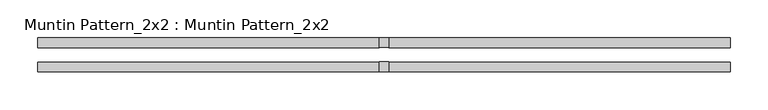
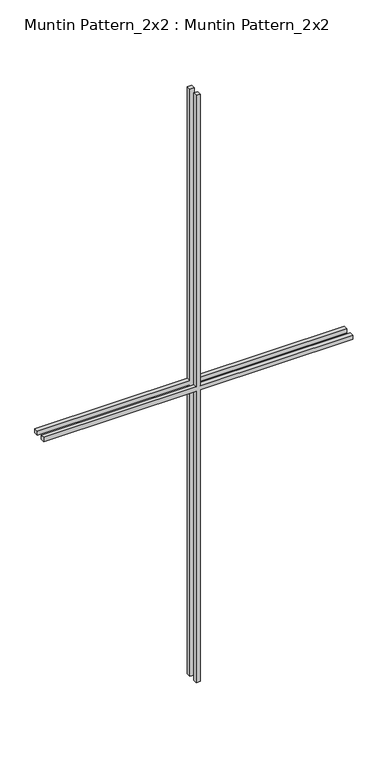
"""IFC4 building model written with IfcOpenShell, lengths in millimetres: proxy geometry, Muntin Pattern_2x2 : Muntin Pattern_2x2."""

from ifc_helpers import new_model, si_unit, frame, origin, place, context, project, spatial, polyline, outline, extrude, source, transform, mapped, element, save


def muntin_pattern_2x2_muntin_pattern_2x2_51cb8927(model_context):
    return source(origin(), model_context, "Body", "SweptSolid", [
        extrude(outline(polyline([(923.925, -6.35), (923.925, -457.2), (911.225, -457.2), (911.225, -6.35), (0.0, -6.35), (0.0, 6.35), (911.225, 6.35), (911.225, 457.2), (923.925, 457.2), (923.925, 6.35), (1835.15, 6.35), (1835.15, -6.35), (923.925, -6.35)])), frame((0.0, 9.525, 0.0), z_axis=(0.0, 1.0, 0.0), x_axis=(0.0, 0.0, 1.0)), (0.0, 0.0, 1.0), 12.7),
        extrude(outline(polyline([(923.925, -6.35), (923.925, -457.2), (911.225, -457.2), (911.225, -6.35), (0.0, -6.35), (0.0, 6.35), (911.225, 6.35), (911.225, 457.2), (923.925, 457.2), (923.925, 6.35), (1835.15, 6.35), (1835.15, -6.35), (923.925, -6.35)])), frame((0.0, -22.225, 0.0), z_axis=(0.0, 1.0, 0.0), x_axis=(0.0, 0.0, 1.0)), (0.0, 0.0, 1.0), 12.7),
    ])


if __name__ == "__main__":
    model = new_model("IFC4")
    model_context = context("Model", 3, world=origin())
    ifc_project = project(units=[si_unit("LENGTHUNIT", "METRE", prefix="MILLI")], contexts=[model_context])
    site = spatial("IfcSite", under=ifc_project)
    building = spatial("IfcBuilding", under=site)
    placement = place(None, origin())
    muntin_pattern_2x2_muntin_pattern_2x2_shape = muntin_pattern_2x2_muntin_pattern_2x2_51cb8927(model_context)
    element("IfcBuildingElementProxy", 1, Name="Muntin Pattern_2x2 : Muntin Pattern_2x2", ObjectType="Muntin Pattern_2x2 : Muntin Pattern_2x2", at=placement, inside=building, context=model_context, shape_type="MappedRepresentation", body=[
        mapped(muntin_pattern_2x2_muntin_pattern_2x2_shape, transform((0.0, 0.0, 0.0), x_axis=(1.0, 0.0, 0.0), y_axis=(0.0, 1.0, 0.0), z_axis=(0.0, 0.0, 1.0))),
    ])
    save(model, "model.ifc")

# Revit data of these elements
# Type "Muntin Pattern_2x2 : Muntin Pattern_2x2"
#   Width [instance default] = 4 ft
#   Thickness = 0.041667 ft
#   Height [instance default] = 4 ft
#   Distance = 0.0625 ft
#   Interior Material [instance default] = none
#   Exterior Material [instance default] = none
#   Default Elevation = 0
# Element 1 (IfcBuildingElementProxy, "Muntin Pattern_2x2 : Muntin Pattern_2x2")
#   Width = 3 ft
#   Height = 6.020833 ft
#   Interior Material = Wood - Stained
#   Exterior Material = Clad - White
#   Materials on its faces: "Clad - White", "Wood - Stained"
# Materials
#   "Clad - White": class "Wood", colour RGB 242 242 238, transparency 0, Cost = 0
#   "Wood - Stained": class "Wood", colour RGB 224 178 126, transparency 0, Cost = 0
